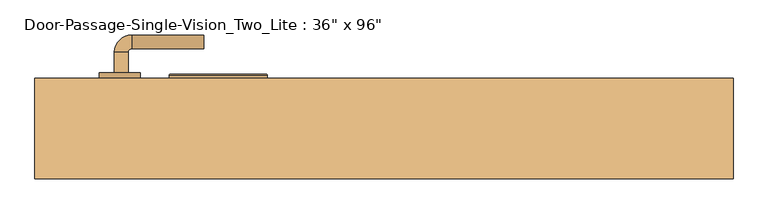
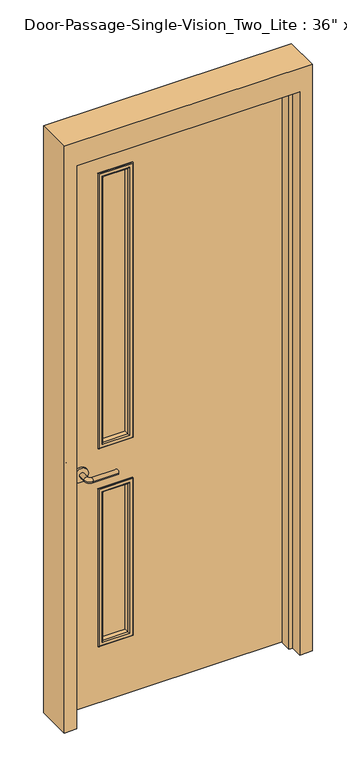
"""IFC4 building model written with IfcOpenShell, lengths in millimetres: door geometry."""

from ifc_helpers import new_model, si_unit, point, frame, frame_2d, origin, place, context, project, spatial, polyline, circle_curve, ellipse_curve, trimmed, segment, composite_curve, outline, extrude, faceted_brep, source, transform, mapped, element, save
from ifc_brep_helpers import plane_surface, cylinder_surface, revolved_surface, advanced_brep


def door_81f4c142(model_context):
    return source(origin(), model_context, "Body", "SolidModel", [
        advanced_brep(
        [(-392.190625, 28.5, 1016.0), (-372.190625, 28.5, 1016.0), (-372.190625, -1.5, 1016.0), (-392.190625, -1.5, 1016.0), (-367.190625, -6.5, 1016.0), (-367.190625, -26.5, 1016.0), (-262.190625, -26.5, 1016.0), (-262.190625, -6.5, 1016.0)],
        [
            (0, 1, circle_curve(frame((-382.190625, 28.5, 1016.0), z_axis=(0.0, 1.0, 0.0), x_axis=(1.0, 0.0, 0.0)), 10.0)),
            (1, 0, circle_curve(frame((-382.190625, 28.5, 1016.0), z_axis=(0.0, 1.0, 0.0), x_axis=(1.0, 0.0, 0.0)), 10.0)),
            (1, 2),
            (2, 3, circle_curve(frame((-382.190625, -1.5, 1016.0), z_axis=(0.0, 1.0, 0.0), x_axis=(1.0, 0.0, 0.0)), 10.0)),
            (3, 0),
            (3, 2, circle_curve(frame((-382.190625, -1.5, 1016.0), z_axis=(0.0, 1.0, 0.0), x_axis=(1.0, 0.0, 0.0)), 10.0)),
            (4, 5, circle_curve(frame((-367.190625, -16.5, 1016.0), z_axis=(-1.0, 0.0, 0.0), x_axis=(0.0, 1.0, 0.0)), 10.0)),
            (5, 3, circle_curve(frame((-367.190625, -1.5, 1016.0), z_axis=(0.0, 0.0, -1.0), x_axis=(-1.0, 0.0, 0.0)), 25.0)),
            (2, 4, circle_curve(frame((-367.190625, -1.5, 1016.0), z_axis=(0.0, 0.0, 1.0), x_axis=(-1.0, 0.0, 0.0)), 5.0)),
            (5, 4, circle_curve(frame((-367.190625, -16.5, 1016.0), z_axis=(-1.0, 0.0, 0.0), x_axis=(0.0, 1.0, 0.0)), 10.0)),
            (6, 7, circle_curve(frame((-262.190625, -16.5, 1016.0), z_axis=(1.0, 0.0, 0.0), x_axis=(0.0, 1.0, 0.0)), 10.0)),
            (7, 6, circle_curve(frame((-262.190625, -16.5, 1016.0), z_axis=(1.0, 0.0, 0.0), x_axis=(0.0, 1.0, 0.0)), 10.0)),
            (4, 7),
            (6, 5),
        ],
        [
            plane_surface(frame((-382.190625, 28.5, 1016.0), z_axis=(0.0, 1.0, 0.0), x_axis=(0.0, 0.0, 1.0))),
            cylinder_surface(frame((-382.190625, 28.5, 1016.0), z_axis=(0.0, 1.0, 0.0), x_axis=(1.0, 0.0, 0.0)), 10.0),
            revolved_surface(trimmed(ellipse_curve(frame((-382.190625, -1.5, 1016.0), z_axis=(0.0, -1.0, 0.0), x_axis=(1.0, 0.0, 0.0)), 10.0, 10.0), [point((-392.190625, -1.5, 1016.0))], [point((-372.190625, -1.5, 1016.0))], True, "CARTESIAN"), (-367.190625, -1.5, 1016.0), (0.0, 0.0, -1.0)),
            revolved_surface(trimmed(ellipse_curve(frame((-382.190625, -1.5, 1016.0), z_axis=(0.0, -1.0, 0.0), x_axis=(1.0, 0.0, 0.0)), 10.0, 10.0), [point((-372.190625, -1.5, 1016.0))], [point((-392.190625, -1.5, 1016.0))], True, "CARTESIAN"), (-367.190625, -1.5, 1016.0), (0.0, 0.0, -1.0)),
            plane_surface(frame((-262.190625, -16.5, 1016.0), z_axis=(1.0, 0.0, 0.0), x_axis=(0.0, 0.0, 1.0))),
            cylinder_surface(frame((-367.190625, -16.5, 1016.0), z_axis=(-1.0, 0.0, 0.0), x_axis=(0.0, 1.0, 0.0)), 10.0),
        ],
        [
            (0, [[1, 2]]),
            (1, [[3, 4, 5, -2]]),
            (1, [[-5, 6, -3, -1]]),
            (2, [[7, 8, -4, 9]]),
            (3, [[10, -9, -6, -8]]),
            (4, [[11, 12]]),
            (5, [[13, -11, 14, -7]]),
            (5, [[-14, -12, -13, -10]]),
        ],
    ),
        extrude(outline(composite_curve([segment(trimmed(circle_curve(frame_2d((1016.0, -384.690625)), 30.0), [point((1016.0, -414.690625))], [point((1016.0, -354.690625))], False, "CARTESIAN"), True, "CONTINUOUS"), segment(trimmed(circle_curve(frame_2d((1016.0, -384.690625)), 30.0), [point((1016.0, -354.690625))], [point((1016.0, -414.690625))], False, "CARTESIAN"), True, "CONTINUOUS")], self_intersect=False)), frame((0.0, 28.5, 0.0), z_axis=(0.0, 1.0, 0.0), x_axis=(0.0, 0.0, 1.0)), (0.0, 0.0, 1.0), 8.0),
        advanced_brep(
        [(-392.190625, 88.95, 1016.0), (-372.190625, 88.95, 1016.0), (-392.190625, 118.95, 1016.0), (-372.190625, 118.95, 1016.0), (-367.190625, 123.95, 1016.0), (-367.190625, 143.95, 1016.0), (-262.190625, 143.95, 1016.0), (-262.190625, 123.95, 1016.0)],
        [
            (0, 1, circle_curve(frame((-382.190625, 88.95, 1016.0), z_axis=(0.0, -1.0, 0.0), x_axis=(1.0, 0.0, 0.0)), 10.0)),
            (1, 0, circle_curve(frame((-382.190625, 88.95, 1016.0), z_axis=(0.0, -1.0, 0.0), x_axis=(1.0, 0.0, 0.0)), 10.0)),
            (0, 2),
            (2, 3, circle_curve(frame((-382.190625, 118.95, 1016.0), z_axis=(0.0, -1.0, 0.0), x_axis=(1.0, 0.0, 0.0)), 10.0)),
            (3, 1),
            (3, 2, circle_curve(frame((-382.190625, 118.95, 1016.0), z_axis=(0.0, -1.0, 0.0), x_axis=(1.0, 0.0, 0.0)), 10.0)),
            (4, 3, circle_curve(frame((-367.190625, 118.95, 1016.0), z_axis=(0.0, 0.0, 1.0), x_axis=(-1.0, 0.0, 0.0)), 5.0)),
            (2, 5, circle_curve(frame((-367.190625, 118.95, 1016.0), z_axis=(0.0, 0.0, -1.0), x_axis=(-1.0, 0.0, 0.0)), 25.0)),
            (5, 4, circle_curve(frame((-367.190625, 133.95, 1016.0), z_axis=(-1.0, 0.0, 0.0), x_axis=(0.0, -1.0, 0.0)), 10.0)),
            (4, 5, circle_curve(frame((-367.190625, 133.95, 1016.0), z_axis=(-1.0, 0.0, 0.0), x_axis=(0.0, -1.0, 0.0)), 10.0)),
            (6, 7, circle_curve(frame((-262.190625, 133.95, 1016.0), z_axis=(1.0, 0.0, 0.0), x_axis=(0.0, -1.0, 0.0)), 10.0)),
            (7, 6, circle_curve(frame((-262.190625, 133.95, 1016.0), z_axis=(1.0, 0.0, 0.0), x_axis=(0.0, -1.0, 0.0)), 10.0)),
            (5, 6),
            (7, 4),
        ],
        [
            plane_surface(frame((-382.190625, 88.95, 1016.0), z_axis=(0.0, -1.0, 0.0), x_axis=(0.0, 0.0, 1.0))),
            cylinder_surface(frame((-382.190625, 88.95, 1016.0), z_axis=(0.0, -1.0, 0.0), x_axis=(1.0, 0.0, 0.0)), 10.0),
            revolved_surface(trimmed(ellipse_curve(frame((-382.190625, 118.95, 1016.0), z_axis=(0.0, -1.0, 0.0), x_axis=(1.0, 0.0, 0.0)), 10.0, 10.0), [point((-392.190625, 118.95, 1016.0))], [point((-372.190625, 118.95, 1016.0))], True, "CARTESIAN"), (-367.190625, 118.95, 1016.0), (0.0, 0.0, -1.0)),
            revolved_surface(trimmed(ellipse_curve(frame((-382.190625, 118.95, 1016.0), z_axis=(0.0, -1.0, 0.0), x_axis=(1.0, 0.0, 0.0)), 10.0, 10.0), [point((-372.190625, 118.95, 1016.0))], [point((-392.190625, 118.95, 1016.0))], True, "CARTESIAN"), (-367.190625, 118.95, 1016.0), (0.0, 0.0, -1.0)),
            plane_surface(frame((-262.190625, 133.95, 1016.0), z_axis=(1.0, 0.0, 0.0), x_axis=(0.0, 0.0, 1.0))),
            cylinder_surface(frame((-367.190625, 133.95, 1016.0), z_axis=(-1.0, 0.0, 0.0), x_axis=(0.0, -1.0, 0.0)), 10.0),
        ],
        [
            (0, [[1, 2]]),
            (1, [[-1, 3, 4, 5]]),
            (1, [[-2, -5, 6, -3]]),
            (2, [[7, -4, 8, 9]]),
            (3, [[-8, -6, -7, 10]]),
            (4, [[11, 12]]),
            (5, [[-9, 13, -12, 14]]),
            (5, [[-10, -14, -11, -13]]),
        ],
    ),
        extrude(outline(composite_curve([segment(trimmed(circle_curve(frame_2d((1016.0, -384.690625)), 30.0), [point((1016.0, -414.690625))], [point((1016.0, -354.690625))], False, "CARTESIAN"), True, "CONTINUOUS"), segment(trimmed(circle_curve(frame_2d((1016.0, -384.690625)), 30.0), [point((1016.0, -354.690625))], [point((1016.0, -414.690625))], False, "CARTESIAN"), True, "CONTINUOUS")], self_intersect=False)), frame((0.0, 80.95, 0.0), z_axis=(0.0, 1.0, 0.0), x_axis=(0.0, 0.0, 1.0)), (0.0, 0.0, 1.0), 8.0),
        faceted_brep([(457.2, 31.7375, 0.0), (457.2, 80.95, 0.0), (508.0, 80.95, 0.0), (508.0, -65.1, 0.0), (457.2, -65.1, 0.0), (457.2, -15.8875, 0.0), (441.325, -15.8875, 0.0), (441.325, 31.7375, 0.0), (457.2, 31.7375, 2438.4), (457.2, 80.95, 2438.4), (-457.2, 80.95, 2438.4), (-457.2, 80.95, 0.0), (-508.0, 80.95, 0.0), (-508.0, 80.95, 2540.0), (508.0, 80.95, 2540.0), (508.0, -65.1, 2540.0), (-508.0, -65.1, 2540.0), (-508.0, -65.1, 0.0), (-457.2, -65.1, 0.0), (-457.2, -65.1, 2438.4), (457.2, -65.1, 2438.4), (457.2, -15.8875, 2438.4), (-457.2, -15.8875, 2438.4), (-457.2, -15.8875, 0.0), (-441.325, -15.8875, 0.0), (-441.325, -15.8875, 2422.525), (441.325, -15.8875, 2422.525), (441.325, 31.7375, 2422.525), (-441.325, 31.7375, 2422.525), (-441.325, 31.7375, 0.0), (-457.2, 31.7375, 0.0), (-457.2, 31.7375, 2438.4)], [[[0, 1, 2, 3, 4, 5, 6, 7]], [[1, 0, 8, 9]], [[2, 1, 9, 10, 11, 12, 13, 14]], [[3, 2, 14, 15]], [[4, 3, 15, 16, 17, 18, 19, 20]], [[5, 4, 20, 21]], [[6, 5, 21, 22, 23, 24, 25, 26]], [[7, 6, 26, 27]], [[0, 7, 27, 28, 29, 30, 31, 8]], [[9, 8, 31, 10]], [[20, 19, 22, 21]], [[26, 25, 28, 27]], [[12, 11, 30, 29, 24, 23, 18, 17]], [[11, 10, 31, 30]], [[13, 12, 17, 16]], [[19, 18, 23, 22]], [[25, 24, 29, 28]], [[15, 14, 13, 16]]]),
        extrude(outline(polyline([(2438.4, -457.2), (0.0, -457.2), (0.0, 457.2), (2438.4, 457.2), (2438.4, -457.2)]), holes=[polyline([(2286.0, -304.8), (2286.0, -177.8), (1111.25, -177.8), (1111.25, -304.8), (2286.0, -304.8)]), polyline([(920.75, -304.8), (920.75, -177.8), (254.0, -177.8), (254.0, -304.8), (920.75, -304.8)])]), frame((0.0, 36.5, 0.0), z_axis=(0.0, 1.0, 0.0), x_axis=(0.0, 0.0, 1.0)), (0.0, 0.0, 1.0), 44.45),
        extrude(outline(polyline([(-177.8, 55.55), (-304.8, 55.55), (-304.8, 61.9), (-177.8, 61.9), (-177.8, 55.55)])), frame((0.0, 0.0, 1111.25), z_axis=(0.0, 0.0, 1.0), x_axis=(1.0, 0.0, 0.0)), (0.0, 0.0, 1.0), 1174.75),
        extrude(outline(polyline([(-177.8, 55.55), (-304.8, 55.55), (-304.8, 61.9), (-177.8, 61.9), (-177.8, 55.55)])), frame((0.0, 0.0, 254.0), z_axis=(0.0, 0.0, 1.0), x_axis=(1.0, 0.0, 0.0)), (0.0, 0.0, 1.0), 666.75),
        advanced_brep(
        [(-177.8, 55.55, 920.75), (-177.8, 36.5, 920.75), (-177.8, 36.5, 254.0), (-177.8, 55.55, 254.0), (-189.8, 35.5, 908.75), (-189.8, 55.55, 908.75), (-189.8, 55.55, 266.0), (-189.8, 35.5, 266.0), (-184.8, 30.5, 913.75), (-184.8, 30.5, 261.0), (-169.8, 32.5, 928.75), (-171.8, 30.5, 926.75), (-171.8, 30.5, 248.0), (-169.8, 32.5, 246.0), (-169.8, 36.5, 928.75), (-169.8, 36.5, 246.0), (-304.8, 36.5, 254.0), (-304.8, 55.55, 254.0), (-292.8, 55.55, 266.0), (-292.8, 35.5, 266.0), (-297.8, 30.5, 261.0), (-310.8, 30.5, 248.0), (-312.8, 32.5, 246.0), (-312.8, 36.5, 246.0), (-304.8, 36.5, 920.75), (-304.8, 55.55, 920.75), (-292.8, 55.55, 908.75), (-292.8, 35.5, 908.75), (-297.8, 30.5, 913.75), (-310.8, 30.5, 926.75), (-312.8, 32.5, 928.75), (-312.8, 36.5, 928.75)],
        [
            (0, 1),
            (1, 2),
            (2, 3),
            (3, 0),
            (4, 5),
            (5, 6),
            (6, 7),
            (7, 4),
            (8, 4, ellipse_curve(frame((-184.8, 35.5, 913.75), z_axis=(0.7071067811865475, 0.0, -0.7071067811865475), x_axis=(0.7071067811865474, 0.0, 0.7071067811865476)), 7.0710678, 5.0)),
            (7, 9, ellipse_curve(frame((-184.8, 35.5, 261.0), z_axis=(0.7071067811865475, 0.0, 0.7071067811865475), x_axis=(-0.7071067811865474, 0.0, 0.7071067811865476)), 7.0710678, 5.0)),
            (9, 8),
            (10, 11, ellipse_curve(frame((-171.8, 32.5, 926.75), z_axis=(0.7071067811865475, 0.0, -0.7071067811865475), x_axis=(0.7071067811865474, 0.0, 0.7071067811865476)), 2.8284271, 2.0)),
            (11, 12),
            (12, 13, ellipse_curve(frame((-171.8, 32.5, 248.0), z_axis=(0.7071067811865475, 0.0, 0.7071067811865475), x_axis=(-0.7071067811865474, 0.0, 0.7071067811865476)), 2.8284271, 2.0)),
            (13, 10),
            (14, 10),
            (13, 15),
            (15, 14),
            (2, 16),
            (16, 17),
            (17, 3),
            (6, 18),
            (18, 19),
            (19, 7),
            (19, 20, ellipse_curve(frame((-297.8, 35.5, 261.0), z_axis=(0.7071067811865475, 0.0, -0.7071067811865475), x_axis=(0.7071067811865476, 0.0, 0.7071067811865474)), 7.0710678, 5.0)),
            (20, 9),
            (12, 21),
            (21, 22, ellipse_curve(frame((-310.8, 32.5, 248.0), z_axis=(0.7071067811865475, 0.0, -0.7071067811865475), x_axis=(0.7071067811865476, 0.0, 0.7071067811865474)), 2.8284271, 2.0)),
            (22, 13),
            (22, 23),
            (23, 15),
            (16, 24),
            (24, 25),
            (25, 17),
            (18, 26),
            (26, 27),
            (27, 19),
            (27, 28, ellipse_curve(frame((-297.8, 35.5, 913.75), z_axis=(-0.7071067811865475, 0.0, -0.7071067811865475), x_axis=(0.7071067811865474, 0.0, -0.7071067811865476)), 7.0710678, 5.0)),
            (28, 20),
            (21, 29),
            (29, 30, ellipse_curve(frame((-310.8, 32.5, 926.75), z_axis=(-0.7071067811865475, 0.0, -0.7071067811865475), x_axis=(0.7071067811865474, 0.0, -0.7071067811865476)), 2.8284271, 2.0)),
            (30, 22),
            (30, 31),
            (31, 23),
            (31, 14),
            (1, 24),
            (0, 25),
            (5, 26),
            (4, 27),
            (8, 28),
            (11, 29),
            (10, 30),
        ],
        [
            plane_surface(frame((-177.8, 36.5, 920.75), z_axis=(1.0, 0.0, 0.0), x_axis=(0.0, 0.0, -1.0))),
            plane_surface(frame((-189.8, 55.55, 908.75), z_axis=(-1.0, 0.0, 0.0), x_axis=(0.0, 0.0, -1.0))),
            cylinder_surface(frame((-184.8, 35.5, 920.75), z_axis=(0.0, 0.0, 1.0), x_axis=(1.0, 0.0, 0.0)), 5.0),
            cylinder_surface(frame((-171.8, 32.5, 920.75), z_axis=(0.0, 0.0, 1.0), x_axis=(1.0, 0.0, 0.0)), 2.0),
            plane_surface(frame((-169.8, 32.5, 928.75), z_axis=(1.0, 0.0, 0.0), x_axis=(0.0, 0.0, -1.0))),
            plane_surface(frame((-177.8, 36.5, 254.0), z_axis=(0.0, 0.0, -1.0), x_axis=(-1.0, 0.0, 0.0))),
            plane_surface(frame((-189.8, 55.55, 266.0), z_axis=(0.0, 0.0, 1.0), x_axis=(-1.0, 0.0, 0.0))),
            cylinder_surface(frame((-177.8, 35.5, 261.0), z_axis=(1.0, 0.0, 0.0), x_axis=(0.0, 0.0, -1.0)), 5.0),
            cylinder_surface(frame((-177.8, 32.5, 248.0), z_axis=(1.0, 0.0, 0.0), x_axis=(0.0, 0.0, -1.0)), 2.0),
            plane_surface(frame((-169.8, 32.5, 246.0), z_axis=(0.0, 0.0, -1.0), x_axis=(-1.0, 0.0, 0.0))),
            plane_surface(frame((-304.8, 36.5, 254.0), z_axis=(-1.0, 0.0, 0.0), x_axis=(0.0, 0.0, 1.0))),
            plane_surface(frame((-292.8, 55.55, 266.0), z_axis=(1.0, 0.0, 0.0), x_axis=(0.0, 0.0, 1.0))),
            cylinder_surface(frame((-297.8, 35.5, 254.0), z_axis=(0.0, 0.0, -1.0), x_axis=(-1.0, 0.0, 0.0)), 5.0),
            cylinder_surface(frame((-310.8, 32.5, 254.0), z_axis=(0.0, 0.0, -1.0), x_axis=(-1.0, 0.0, 0.0)), 2.0),
            plane_surface(frame((-312.8, 32.5, 246.0), z_axis=(-1.0, 0.0, 0.0), x_axis=(0.0, 0.0, 1.0))),
            plane_surface(frame((-312.8, 36.5, 928.75), z_axis=(0.0, 1.0, 0.0), x_axis=(1.0, 0.0, 0.0))),
            plane_surface(frame((-304.8, 36.5, 920.75), z_axis=(0.0, 0.0, 1.0), x_axis=(1.0, 0.0, 0.0))),
            plane_surface(frame((-304.8, 55.55, 920.75), z_axis=(0.0, 1.0, 0.0), x_axis=(1.0, 0.0, 0.0))),
            plane_surface(frame((-292.8, 55.55, 908.75), z_axis=(0.0, 0.0, -1.0), x_axis=(1.0, 0.0, 0.0))),
            cylinder_surface(frame((-304.8, 35.5, 913.75), z_axis=(-1.0, 0.0, 0.0), x_axis=(0.0, 0.0, 1.0)), 5.0),
            plane_surface(frame((-297.8, 30.5, 913.75), z_axis=(0.0, -1.0, 0.0), x_axis=(1.0, 0.0, 0.0))),
            cylinder_surface(frame((-304.8, 32.5, 926.75), z_axis=(-1.0, 0.0, 0.0), x_axis=(0.0, 0.0, 1.0)), 2.0),
            plane_surface(frame((-312.8, 32.5, 928.75), z_axis=(0.0, 0.0, 1.0), x_axis=(1.0, 0.0, 0.0))),
        ],
        [
            (0, [[1, 2, 3, 4]]),
            (1, [[5, 6, 7, 8]]),
            (2, [[9, -8, 10, 11]]),
            (3, [[12, 13, 14, 15]]),
            (4, [[16, -15, 17, 18]]),
            (5, [[-3, 19, 20, 21]]),
            (6, [[-7, 22, 23, 24]]),
            (7, [[-10, -24, 25, 26]]),
            (8, [[-14, 27, 28, 29]]),
            (9, [[-17, -29, 30, 31]]),
            (10, [[-20, 32, 33, 34]]),
            (11, [[-23, 35, 36, 37]]),
            (12, [[-25, -37, 38, 39]]),
            (13, [[-28, 40, 41, 42]]),
            (14, [[-30, -42, 43, 44]]),
            (15, [[-31, -44, 45, -18], [46, -32, -19, -2]]),
            (16, [[-33, -46, -1, 47]]),
            (17, [[-21, -34, -47, -4], [48, -35, -22, -6]]),
            (18, [[-36, -48, -5, 49]]),
            (19, [[-38, -49, -9, 50]]),
            (20, [[51, -40, -27, -13], [-26, -39, -50, -11]]),
            (21, [[-41, -51, -12, 52]]),
            (22, [[-43, -52, -16, -45]]),
        ],
    ),
        advanced_brep(
        [(-304.8, 61.9, 920.75), (-304.8, 80.95, 920.75), (-304.8, 80.95, 254.0), (-304.8, 61.9, 254.0), (-292.8, 81.95, 908.75), (-292.8, 61.9, 908.75), (-292.8, 61.9, 266.0), (-292.8, 81.95, 266.0), (-297.8, 86.95, 913.75), (-297.8, 86.95, 261.0), (-312.8, 84.95, 928.75), (-310.8, 86.95, 926.75), (-310.8, 86.95, 248.0), (-312.8, 84.95, 246.0), (-312.8, 80.95, 928.75), (-312.8, 80.95, 246.0), (-177.8, 80.95, 254.0), (-177.8, 61.9, 254.0), (-189.8, 61.9, 266.0), (-189.8, 81.95, 266.0), (-184.8, 86.95, 261.0), (-171.8, 86.95, 248.0), (-169.8, 84.95, 246.0), (-169.8, 80.95, 246.0), (-177.8, 80.95, 920.75), (-177.8, 61.9, 920.75), (-189.8, 61.9, 908.75), (-189.8, 81.95, 908.75), (-184.8, 86.95, 913.75), (-171.8, 86.95, 926.75), (-169.8, 84.95, 928.75), (-169.8, 80.95, 928.75)],
        [
            (0, 1),
            (1, 2),
            (2, 3),
            (3, 0),
            (4, 5),
            (5, 6),
            (6, 7),
            (7, 4),
            (8, 4, ellipse_curve(frame((-297.8, 81.95, 913.75), z_axis=(-0.7071067811865475, 0.0, -0.7071067811865475), x_axis=(-0.7071067811865474, 0.0, 0.7071067811865476)), 7.0710678, 5.0)),
            (7, 9, ellipse_curve(frame((-297.8, 81.95, 261.0), z_axis=(-0.7071067811865475, 0.0, 0.7071067811865475), x_axis=(0.7071067811865474, 0.0, 0.7071067811865476)), 7.0710678, 5.0)),
            (9, 8),
            (10, 11, ellipse_curve(frame((-310.8, 84.95, 926.75), z_axis=(-0.7071067811865475, 0.0, -0.7071067811865475), x_axis=(-0.7071067811865474, 0.0, 0.7071067811865476)), 2.8284271, 2.0)),
            (11, 12),
            (12, 13, ellipse_curve(frame((-310.8, 84.95, 248.0), z_axis=(-0.7071067811865475, 0.0, 0.7071067811865475), x_axis=(0.7071067811865474, 0.0, 0.7071067811865476)), 2.8284271, 2.0)),
            (13, 10),
            (14, 10),
            (13, 15),
            (15, 14),
            (2, 16),
            (16, 17),
            (17, 3),
            (6, 18),
            (18, 19),
            (19, 7),
            (19, 20, ellipse_curve(frame((-184.8, 81.95, 261.0), z_axis=(-0.7071067811865475, 0.0, -0.7071067811865475), x_axis=(-0.7071067811865476, 0.0, 0.7071067811865474)), 7.0710678, 5.0)),
            (20, 9),
            (12, 21),
            (21, 22, ellipse_curve(frame((-171.8, 84.95, 248.0), z_axis=(-0.7071067811865475, 0.0, -0.7071067811865475), x_axis=(-0.7071067811865476, 0.0, 0.7071067811865474)), 2.8284271, 2.0)),
            (22, 13),
            (22, 23),
            (23, 15),
            (16, 24),
            (24, 25),
            (25, 17),
            (18, 26),
            (26, 27),
            (27, 19),
            (27, 28, ellipse_curve(frame((-184.8, 81.95, 913.75), z_axis=(0.7071067811865475, 0.0, -0.7071067811865475), x_axis=(-0.7071067811865474, 0.0, -0.7071067811865476)), 7.0710678, 5.0)),
            (28, 20),
            (21, 29),
            (29, 30, ellipse_curve(frame((-171.8, 84.95, 926.75), z_axis=(0.7071067811865475, 0.0, -0.7071067811865475), x_axis=(-0.7071067811865474, 0.0, -0.7071067811865476)), 2.8284271, 2.0)),
            (30, 22),
            (30, 31),
            (31, 23),
            (31, 14),
            (1, 24),
            (0, 25),
            (5, 26),
            (4, 27),
            (8, 28),
            (11, 29),
            (10, 30),
        ],
        [
            plane_surface(frame((-304.8, 80.95, 920.75), z_axis=(-1.0, 0.0, 0.0), x_axis=(0.0, 0.0, -1.0))),
            plane_surface(frame((-292.8, 61.9, 908.75), z_axis=(1.0, 0.0, 0.0), x_axis=(0.0, 0.0, -1.0))),
            cylinder_surface(frame((-297.8, 81.95, 920.75), z_axis=(0.0, 0.0, 1.0), x_axis=(-1.0, 0.0, 0.0)), 5.0),
            cylinder_surface(frame((-310.8, 84.95, 920.75), z_axis=(0.0, 0.0, 1.0), x_axis=(-1.0, 0.0, 0.0)), 2.0),
            plane_surface(frame((-312.8, 84.95, 928.75), z_axis=(-1.0, 0.0, 0.0), x_axis=(0.0, 0.0, -1.0))),
            plane_surface(frame((-304.8, 80.95, 254.0), z_axis=(0.0, 0.0, -1.0), x_axis=(1.0, 0.0, 0.0))),
            plane_surface(frame((-292.8, 61.9, 266.0), z_axis=(0.0, 0.0, 1.0), x_axis=(1.0, 0.0, 0.0))),
            cylinder_surface(frame((-304.8, 81.95, 261.0), z_axis=(-1.0, 0.0, 0.0), x_axis=(0.0, 0.0, -1.0)), 5.0),
            cylinder_surface(frame((-304.8, 84.95, 248.0), z_axis=(-1.0, 0.0, 0.0), x_axis=(0.0, 0.0, -1.0)), 2.0),
            plane_surface(frame((-312.8, 84.95, 246.0), z_axis=(0.0, 0.0, -1.0), x_axis=(1.0, 0.0, 0.0))),
            plane_surface(frame((-177.8, 80.95, 254.0), z_axis=(1.0, 0.0, 0.0), x_axis=(0.0, 0.0, 1.0))),
            plane_surface(frame((-189.8, 61.9, 266.0), z_axis=(-1.0, 0.0, 0.0), x_axis=(0.0, 0.0, 1.0))),
            cylinder_surface(frame((-184.8, 81.95, 254.0), z_axis=(0.0, 0.0, -1.0), x_axis=(1.0, 0.0, 0.0)), 5.0),
            cylinder_surface(frame((-171.8, 84.95, 254.0), z_axis=(0.0, 0.0, -1.0), x_axis=(1.0, 0.0, 0.0)), 2.0),
            plane_surface(frame((-169.8, 84.95, 246.0), z_axis=(1.0, 0.0, 0.0), x_axis=(0.0, 0.0, 1.0))),
            plane_surface(frame((-169.8, 80.95, 928.75), z_axis=(0.0, -1.0, 0.0), x_axis=(-1.0, 0.0, 0.0))),
            plane_surface(frame((-177.8, 80.95, 920.75), z_axis=(0.0, 0.0, 1.0), x_axis=(-1.0, 0.0, 0.0))),
            plane_surface(frame((-177.8, 61.9, 920.75), z_axis=(0.0, -1.0, 0.0), x_axis=(-1.0, 0.0, 0.0))),
            plane_surface(frame((-189.8, 61.9, 908.75), z_axis=(0.0, 0.0, -1.0), x_axis=(-1.0, 0.0, 0.0))),
            cylinder_surface(frame((-177.8, 81.95, 913.75), z_axis=(1.0, 0.0, 0.0), x_axis=(0.0, 0.0, 1.0)), 5.0),
            plane_surface(frame((-184.8, 86.95, 913.75), z_axis=(0.0, 1.0, 0.0), x_axis=(-1.0, 0.0, 0.0))),
            cylinder_surface(frame((-177.8, 84.95, 926.75), z_axis=(1.0, 0.0, 0.0), x_axis=(0.0, 0.0, 1.0)), 2.0),
            plane_surface(frame((-169.8, 84.95, 928.75), z_axis=(0.0, 0.0, 1.0), x_axis=(-1.0, 0.0, 0.0))),
        ],
        [
            (0, [[1, 2, 3, 4]]),
            (1, [[5, 6, 7, 8]]),
            (2, [[9, -8, 10, 11]]),
            (3, [[12, 13, 14, 15]]),
            (4, [[16, -15, 17, 18]]),
            (5, [[-3, 19, 20, 21]]),
            (6, [[-7, 22, 23, 24]]),
            (7, [[-10, -24, 25, 26]]),
            (8, [[-14, 27, 28, 29]]),
            (9, [[-17, -29, 30, 31]]),
            (10, [[-20, 32, 33, 34]]),
            (11, [[-23, 35, 36, 37]]),
            (12, [[-25, -37, 38, 39]]),
            (13, [[-28, 40, 41, 42]]),
            (14, [[-30, -42, 43, 44]]),
            (15, [[-31, -44, 45, -18], [46, -32, -19, -2]]),
            (16, [[-33, -46, -1, 47]]),
            (17, [[-21, -34, -47, -4], [48, -35, -22, -6]]),
            (18, [[-36, -48, -5, 49]]),
            (19, [[-38, -49, -9, 50]]),
            (20, [[51, -40, -27, -13], [-26, -39, -50, -11]]),
            (21, [[-41, -51, -12, 52]]),
            (22, [[-43, -52, -16, -45]]),
        ],
    ),
        advanced_brep(
        [(-304.8, 55.55, 1111.25), (-304.8, 36.5, 1111.25), (-304.8, 36.5, 2286.0), (-304.8, 55.55, 2286.0), (-292.8, 35.5, 1123.25), (-292.8, 55.55, 1123.25), (-292.8, 55.55, 2274.0), (-292.8, 35.5, 2274.0), (-297.8, 30.5, 1118.25), (-297.8, 30.5, 2279.0), (-312.8, 32.5, 1103.25), (-310.8, 30.5, 1105.25), (-310.8, 30.5, 2292.0), (-312.8, 32.5, 2294.0), (-312.8, 36.5, 1103.25), (-312.8, 36.5, 2294.0), (-177.8, 36.5, 2286.0), (-177.8, 55.55, 2286.0), (-189.8, 55.55, 2274.0), (-189.8, 35.5, 2274.0), (-184.8, 30.5, 2279.0), (-171.8, 30.5, 2292.0), (-169.8, 32.5, 2294.0), (-169.8, 36.5, 2294.0), (-177.8, 36.5, 1111.25), (-177.8, 55.55, 1111.25), (-189.8, 55.55, 1123.25), (-189.8, 35.5, 1123.25), (-184.8, 30.5, 1118.25), (-171.8, 30.5, 1105.25), (-169.8, 32.5, 1103.25), (-169.8, 36.5, 1103.25)],
        [
            (0, 1),
            (1, 2),
            (2, 3),
            (3, 0),
            (4, 5),
            (5, 6),
            (6, 7),
            (7, 4),
            (8, 4, ellipse_curve(frame((-297.8, 35.5, 1118.25), z_axis=(-0.7071067811865475, 0.0, 0.7071067811865475), x_axis=(-0.7071067811865474, 0.0, -0.7071067811865476)), 7.0710678, 5.0)),
            (7, 9, ellipse_curve(frame((-297.8, 35.5, 2279.0), z_axis=(-0.7071067811865475, 0.0, -0.7071067811865475), x_axis=(0.7071067811865474, 0.0, -0.7071067811865476)), 7.0710678, 5.0)),
            (9, 8),
            (10, 11, ellipse_curve(frame((-310.8, 32.5, 1105.25), z_axis=(-0.7071067811865475, 0.0, 0.7071067811865475), x_axis=(-0.7071067811865474, 0.0, -0.7071067811865476)), 2.8284271, 2.0)),
            (11, 12),
            (12, 13, ellipse_curve(frame((-310.8, 32.5, 2292.0), z_axis=(-0.7071067811865475, 0.0, -0.7071067811865475), x_axis=(0.7071067811865474, 0.0, -0.7071067811865476)), 2.8284271, 2.0)),
            (13, 10),
            (14, 10),
            (13, 15),
            (15, 14),
            (2, 16),
            (16, 17),
            (17, 3),
            (6, 18),
            (18, 19),
            (19, 7),
            (19, 20, ellipse_curve(frame((-184.8, 35.5, 2279.0), z_axis=(-0.7071067811865475, 0.0, 0.7071067811865475), x_axis=(-0.7071067811865476, 0.0, -0.7071067811865474)), 7.0710678, 5.0)),
            (20, 9),
            (12, 21),
            (21, 22, ellipse_curve(frame((-171.8, 32.5, 2292.0), z_axis=(-0.7071067811865475, 0.0, 0.7071067811865475), x_axis=(-0.7071067811865476, 0.0, -0.7071067811865474)), 2.8284271, 2.0)),
            (22, 13),
            (22, 23),
            (23, 15),
            (16, 24),
            (24, 25),
            (25, 17),
            (18, 26),
            (26, 27),
            (27, 19),
            (27, 28, ellipse_curve(frame((-184.8, 35.5, 1118.25), z_axis=(0.7071067811865475, 0.0, 0.7071067811865475), x_axis=(-0.7071067811865474, 0.0, 0.7071067811865476)), 7.0710678, 5.0)),
            (28, 20),
            (21, 29),
            (29, 30, ellipse_curve(frame((-171.8, 32.5, 1105.25), z_axis=(0.7071067811865475, 0.0, 0.7071067811865475), x_axis=(-0.7071067811865474, 0.0, 0.7071067811865476)), 2.8284271, 2.0)),
            (30, 22),
            (30, 31),
            (31, 23),
            (31, 14),
            (1, 24),
            (0, 25),
            (5, 26),
            (4, 27),
            (8, 28),
            (11, 29),
            (10, 30),
        ],
        [
            plane_surface(frame((-304.8, 36.5, 1111.25), z_axis=(-1.0, 0.0, 0.0), x_axis=(0.0, 0.0, 1.0))),
            plane_surface(frame((-292.8, 55.55, 1123.25), z_axis=(1.0, 0.0, 0.0), x_axis=(0.0, 0.0, 1.0))),
            cylinder_surface(frame((-297.8, 35.5, 1111.25), z_axis=(0.0, 0.0, -1.0), x_axis=(-1.0, 0.0, 0.0)), 5.0),
            cylinder_surface(frame((-310.8, 32.5, 1111.25), z_axis=(0.0, 0.0, -1.0), x_axis=(-1.0, 0.0, 0.0)), 2.0),
            plane_surface(frame((-312.8, 32.5, 1103.25), z_axis=(-1.0, 0.0, 0.0), x_axis=(0.0, 0.0, 1.0))),
            plane_surface(frame((-304.8, 36.5, 2286.0), z_axis=(0.0, 0.0, 1.0), x_axis=(1.0, 0.0, 0.0))),
            plane_surface(frame((-292.8, 55.55, 2274.0), z_axis=(0.0, 0.0, -1.0), x_axis=(1.0, 0.0, 0.0))),
            cylinder_surface(frame((-304.8, 35.5, 2279.0), z_axis=(-1.0, 0.0, 0.0), x_axis=(0.0, 0.0, 1.0)), 5.0),
            cylinder_surface(frame((-304.8, 32.5, 2292.0), z_axis=(-1.0, 0.0, 0.0), x_axis=(0.0, 0.0, 1.0)), 2.0),
            plane_surface(frame((-312.8, 32.5, 2294.0), z_axis=(0.0, 0.0, 1.0), x_axis=(1.0, 0.0, 0.0))),
            plane_surface(frame((-177.8, 36.5, 2286.0), z_axis=(1.0, 0.0, 0.0), x_axis=(0.0, 0.0, -1.0))),
            plane_surface(frame((-189.8, 55.55, 2274.0), z_axis=(-1.0, 0.0, 0.0), x_axis=(0.0, 0.0, -1.0))),
            cylinder_surface(frame((-184.8, 35.5, 2286.0), z_axis=(0.0, 0.0, 1.0), x_axis=(1.0, 0.0, 0.0)), 5.0),
            cylinder_surface(frame((-171.8, 32.5, 2286.0), z_axis=(0.0, 0.0, 1.0), x_axis=(1.0, 0.0, 0.0)), 2.0),
            plane_surface(frame((-169.8, 32.5, 2294.0), z_axis=(1.0, 0.0, 0.0), x_axis=(0.0, 0.0, -1.0))),
            plane_surface(frame((-169.8, 36.5, 1103.25), z_axis=(0.0, 1.0, 0.0), x_axis=(-1.0, 0.0, 0.0))),
            plane_surface(frame((-177.8, 36.5, 1111.25), z_axis=(0.0, 0.0, -1.0), x_axis=(-1.0, 0.0, 0.0))),
            plane_surface(frame((-177.8, 55.55, 1111.25), z_axis=(0.0, 1.0, 0.0), x_axis=(-1.0, 0.0, 0.0))),
            plane_surface(frame((-189.8, 55.55, 1123.25), z_axis=(0.0, 0.0, 1.0), x_axis=(-1.0, 0.0, 0.0))),
            cylinder_surface(frame((-177.8, 35.5, 1118.25), z_axis=(1.0, 0.0, 0.0), x_axis=(0.0, 0.0, -1.0)), 5.0),
            plane_surface(frame((-184.8, 30.5, 1118.25), z_axis=(0.0, -1.0, 0.0), x_axis=(-1.0, 0.0, 0.0))),
            cylinder_surface(frame((-177.8, 32.5, 1105.25), z_axis=(1.0, 0.0, 0.0), x_axis=(0.0, 0.0, -1.0)), 2.0),
            plane_surface(frame((-169.8, 32.5, 1103.25), z_axis=(0.0, 0.0, -1.0), x_axis=(-1.0, 0.0, 0.0))),
        ],
        [
            (0, [[1, 2, 3, 4]]),
            (1, [[5, 6, 7, 8]]),
            (2, [[9, -8, 10, 11]]),
            (3, [[12, 13, 14, 15]]),
            (4, [[16, -15, 17, 18]]),
            (5, [[-3, 19, 20, 21]]),
            (6, [[-7, 22, 23, 24]]),
            (7, [[-10, -24, 25, 26]]),
            (8, [[-14, 27, 28, 29]]),
            (9, [[-17, -29, 30, 31]]),
            (10, [[-20, 32, 33, 34]]),
            (11, [[-23, 35, 36, 37]]),
            (12, [[-25, -37, 38, 39]]),
            (13, [[-28, 40, 41, 42]]),
            (14, [[-30, -42, 43, 44]]),
            (15, [[-31, -44, 45, -18], [46, -32, -19, -2]]),
            (16, [[-33, -46, -1, 47]]),
            (17, [[-21, -34, -47, -4], [48, -35, -22, -6]]),
            (18, [[-36, -48, -5, 49]]),
            (19, [[-38, -49, -9, 50]]),
            (20, [[51, -40, -27, -13], [-26, -39, -50, -11]]),
            (21, [[-41, -51, -12, 52]]),
            (22, [[-43, -52, -16, -45]]),
        ],
    ),
        advanced_brep(
        [(-304.8, 61.9, 2286.0), (-304.8, 80.95, 2286.0), (-304.8, 80.95, 1111.25), (-304.8, 61.9, 1111.25), (-292.8, 81.95, 2274.0), (-292.8, 61.9, 2274.0), (-292.8, 61.9, 1123.25), (-292.8, 81.95, 1123.25), (-297.8, 86.95, 2279.0), (-297.8, 86.95, 1118.25), (-312.8, 84.95, 2294.0), (-310.8, 86.95, 2292.0), (-310.8, 86.95, 1105.25), (-312.8, 84.95, 1103.25), (-312.8, 80.95, 2294.0), (-312.8, 80.95, 1103.25), (-177.8, 80.95, 1111.25), (-177.8, 61.9, 1111.25), (-189.8, 61.9, 1123.25), (-189.8, 81.95, 1123.25), (-184.8, 86.95, 1118.25), (-171.8, 86.95, 1105.25), (-169.8, 84.95, 1103.25), (-169.8, 80.95, 1103.25), (-177.8, 80.95, 2286.0), (-177.8, 61.9, 2286.0), (-189.8, 61.9, 2274.0), (-189.8, 81.95, 2274.0), (-184.8, 86.95, 2279.0), (-171.8, 86.95, 2292.0), (-169.8, 84.95, 2294.0), (-169.8, 80.95, 2294.0)],
        [
            (0, 1),
            (1, 2),
            (2, 3),
            (3, 0),
            (4, 5),
            (5, 6),
            (6, 7),
            (7, 4),
            (8, 4, ellipse_curve(frame((-297.8, 81.95, 2279.0), z_axis=(-0.7071067811865475, 0.0, -0.7071067811865475), x_axis=(-0.7071067811865474, 0.0, 0.7071067811865476)), 7.0710678, 5.0)),
            (7, 9, ellipse_curve(frame((-297.8, 81.95, 1118.25), z_axis=(-0.7071067811865475, 0.0, 0.7071067811865475), x_axis=(0.7071067811865474, 0.0, 0.7071067811865476)), 7.0710678, 5.0)),
            (9, 8),
            (10, 11, ellipse_curve(frame((-310.8, 84.95, 2292.0), z_axis=(-0.7071067811865475, 0.0, -0.7071067811865475), x_axis=(-0.7071067811865474, 0.0, 0.7071067811865476)), 2.8284271, 2.0)),
            (11, 12),
            (12, 13, ellipse_curve(frame((-310.8, 84.95, 1105.25), z_axis=(-0.7071067811865475, 0.0, 0.7071067811865475), x_axis=(0.7071067811865474, 0.0, 0.7071067811865476)), 2.8284271, 2.0)),
            (13, 10),
            (14, 10),
            (13, 15),
            (15, 14),
            (2, 16),
            (16, 17),
            (17, 3),
            (6, 18),
            (18, 19),
            (19, 7),
            (19, 20, ellipse_curve(frame((-184.8, 81.95, 1118.25), z_axis=(-0.7071067811865475, 0.0, -0.7071067811865475), x_axis=(-0.7071067811865476, 0.0, 0.7071067811865474)), 7.0710678, 5.0)),
            (20, 9),
            (12, 21),
            (21, 22, ellipse_curve(frame((-171.8, 84.95, 1105.25), z_axis=(-0.7071067811865475, 0.0, -0.7071067811865475), x_axis=(-0.7071067811865476, 0.0, 0.7071067811865474)), 2.8284271, 2.0)),
            (22, 13),
            (22, 23),
            (23, 15),
            (16, 24),
            (24, 25),
            (25, 17),
            (18, 26),
            (26, 27),
            (27, 19),
            (27, 28, ellipse_curve(frame((-184.8, 81.95, 2279.0), z_axis=(0.7071067811865475, 0.0, -0.7071067811865475), x_axis=(-0.7071067811865474, 0.0, -0.7071067811865476)), 7.0710678, 5.0)),
            (28, 20),
            (21, 29),
            (29, 30, ellipse_curve(frame((-171.8, 84.95, 2292.0), z_axis=(0.7071067811865475, 0.0, -0.7071067811865475), x_axis=(-0.7071067811865474, 0.0, -0.7071067811865476)), 2.8284271, 2.0)),
            (30, 22),
            (30, 31),
            (31, 23),
            (31, 14),
            (1, 24),
            (0, 25),
            (5, 26),
            (4, 27),
            (8, 28),
            (11, 29),
            (10, 30),
        ],
        [
            plane_surface(frame((-304.8, 80.95, 2286.0), z_axis=(-1.0, 0.0, 0.0), x_axis=(0.0, 0.0, -1.0))),
            plane_surface(frame((-292.8, 61.9, 2274.0), z_axis=(1.0, 0.0, 0.0), x_axis=(0.0, 0.0, -1.0))),
            cylinder_surface(frame((-297.8, 81.95, 2286.0), z_axis=(0.0, 0.0, 1.0), x_axis=(-1.0, 0.0, 0.0)), 5.0),
            cylinder_surface(frame((-310.8, 84.95, 2286.0), z_axis=(0.0, 0.0, 1.0), x_axis=(-1.0, 0.0, 0.0)), 2.0),
            plane_surface(frame((-312.8, 84.95, 2294.0), z_axis=(-1.0, 0.0, 0.0), x_axis=(0.0, 0.0, -1.0))),
            plane_surface(frame((-304.8, 80.95, 1111.25), z_axis=(0.0, 0.0, -1.0), x_axis=(1.0, 0.0, 0.0))),
            plane_surface(frame((-292.8, 61.9, 1123.25), z_axis=(0.0, 0.0, 1.0), x_axis=(1.0, 0.0, 0.0))),
            cylinder_surface(frame((-304.8, 81.95, 1118.25), z_axis=(-1.0, 0.0, 0.0), x_axis=(0.0, 0.0, -1.0)), 5.0),
            cylinder_surface(frame((-304.8, 84.95, 1105.25), z_axis=(-1.0, 0.0, 0.0), x_axis=(0.0, 0.0, -1.0)), 2.0),
            plane_surface(frame((-312.8, 84.95, 1103.25), z_axis=(0.0, 0.0, -1.0), x_axis=(1.0, 0.0, 0.0))),
            plane_surface(frame((-177.8, 80.95, 1111.25), z_axis=(1.0, 0.0, 0.0), x_axis=(0.0, 0.0, 1.0))),
            plane_surface(frame((-189.8, 61.9, 1123.25), z_axis=(-1.0, 0.0, 0.0), x_axis=(0.0, 0.0, 1.0))),
            cylinder_surface(frame((-184.8, 81.95, 1111.25), z_axis=(0.0, 0.0, -1.0), x_axis=(1.0, 0.0, 0.0)), 5.0),
            cylinder_surface(frame((-171.8, 84.95, 1111.25), z_axis=(0.0, 0.0, -1.0), x_axis=(1.0, 0.0, 0.0)), 2.0),
            plane_surface(frame((-169.8, 84.95, 1103.25), z_axis=(1.0, 0.0, 0.0), x_axis=(0.0, 0.0, 1.0))),
            plane_surface(frame((-169.8, 80.95, 2294.0), z_axis=(0.0, -1.0, 0.0), x_axis=(-1.0, 0.0, 0.0))),
            plane_surface(frame((-177.8, 80.95, 2286.0), z_axis=(0.0, 0.0, 1.0), x_axis=(-1.0, 0.0, 0.0))),
            plane_surface(frame((-177.8, 61.9, 2286.0), z_axis=(0.0, -1.0, 0.0), x_axis=(-1.0, 0.0, 0.0))),
            plane_surface(frame((-189.8, 61.9, 2274.0), z_axis=(0.0, 0.0, -1.0), x_axis=(-1.0, 0.0, 0.0))),
            cylinder_surface(frame((-177.8, 81.95, 2279.0), z_axis=(1.0, 0.0, 0.0), x_axis=(0.0, 0.0, 1.0)), 5.0),
            plane_surface(frame((-184.8, 86.95, 2279.0), z_axis=(0.0, 1.0, 0.0), x_axis=(-1.0, 0.0, 0.0))),
            cylinder_surface(frame((-177.8, 84.95, 2292.0), z_axis=(1.0, 0.0, 0.0), x_axis=(0.0, 0.0, 1.0)), 2.0),
            plane_surface(frame((-169.8, 84.95, 2294.0), z_axis=(0.0, 0.0, 1.0), x_axis=(-1.0, 0.0, 0.0))),
        ],
        [
            (0, [[1, 2, 3, 4]]),
            (1, [[5, 6, 7, 8]]),
            (2, [[9, -8, 10, 11]]),
            (3, [[12, 13, 14, 15]]),
            (4, [[16, -15, 17, 18]]),
            (5, [[-3, 19, 20, 21]]),
            (6, [[-7, 22, 23, 24]]),
            (7, [[-10, -24, 25, 26]]),
            (8, [[-14, 27, 28, 29]]),
            (9, [[-17, -29, 30, 31]]),
            (10, [[-20, 32, 33, 34]]),
            (11, [[-23, 35, 36, 37]]),
            (12, [[-25, -37, 38, 39]]),
            (13, [[-28, 40, 41, 42]]),
            (14, [[-30, -42, 43, 44]]),
            (15, [[-31, -44, 45, -18], [46, -32, -19, -2]]),
            (16, [[-33, -46, -1, 47]]),
            (17, [[-21, -34, -47, -4], [48, -35, -22, -6]]),
            (18, [[-36, -48, -5, 49]]),
            (19, [[-38, -49, -9, 50]]),
            (20, [[51, -40, -27, -13], [-26, -39, -50, -11]]),
            (21, [[-41, -51, -12, 52]]),
            (22, [[-43, -52, -16, -45]]),
        ],
    ),
    ])


if __name__ == "__main__":
    model = new_model("IFC4")
    model_context = context("Model", 3, world=origin())
    ifc_project = project(units=[si_unit("LENGTHUNIT", "METRE", prefix="MILLI")], contexts=[model_context])
    site = spatial("IfcSite", under=ifc_project)
    building = spatial("IfcBuilding", under=site)
    placement = place(None, origin())
    door_shape = door_81f4c142(model_context)
    element("IfcDoor", 1, ObjectType="Door-Passage-Single-Vision_Two_Lite : 36\" x 96\"", at=placement, inside=building, context=model_context, shape_type="MappedRepresentation", body=[
        mapped(door_shape, transform((0.0, 0.0, 0.0), x_axis=(1.0, 0.0, 0.0), y_axis=(0.0, 1.0, 0.0), z_axis=(0.0, 0.0, 1.0))),
    ])
    save(model, "model.ifc")

# Revit data of these elements
# Type "Door-Passage-Single-Vision_Two_Lite : 36\" x 96\""
#   Type Mark = "22"
#   Assembly Code = "B2030100"
#   Analytic Construction = "Wooden"
#   Thickness = 0' - 1 3/4"
#   Thermal Resistance (R) = 0.455703 (m²·K)/W
#   Swing Angle [instance default] = 90.00°
#   Strike Height = 3' - 4"
#   Rough Width [instance default] = 3' - 4"
#   Rough Height [instance default] = 8' - 4"
#   MF Opening Height [instance default] = 0' - 4"
#   MF Opening Width [instance default] = 0' - 4"
#   Heat Transfer Coefficient (U) = 2.19465 W/(m²·K)
#   Inset Calculate [instance default] = 0' - 4"
#   Masonry Inset [instance default] = 0' - 1"
#   Height = 8' - 0"
#   Width = 3' - 0"
#   Masonry Frame Depth = 0' - 5 3/4"
#   Masonry Frame [instance default] = yes
#   Function = 1
#   Dry Wall Frame [instance default] = no
#   Panel Material = Wood - Birch
#   Glazing = Glass
#   Glass Stop Material = Metal - Paint Finish - Grey
#   Frame Material = Metal - Paint Finish - Grey
#   Door Handle Material = Aluminum
#   Visual Light Transmittance = 0
#   Solar Heat Gain Coefficient = 0
#   Wall Closure = (empty or 0)
# Element 1 (IfcDoor, "Door-Passage-Single-Vision_Two_Lite : 36\" x 96\"")
#   Materials on its faces: "Metal - Paint Finish - Grey", "Aluminum", "Wood - Birch", "Glass"
# Materials
#   "Wood - Birch": class "Wood", colour RGB 166 116 52, transparency 0, Cost = 0
#   "Glass": class "Glass", colour RGB 218 227 224, transparency 0.85, Description = "Soda Lime Glass", Cost = 0
#   "Metal - Paint Finish - Grey": class "Paint", colour RGB 104 104 104, transparency 0, Cost = 0
#   "Aluminum": class "Metal", colour RGB 244 244 244, transparency 0, Description = "Aluminum 6061", Cost = 0
